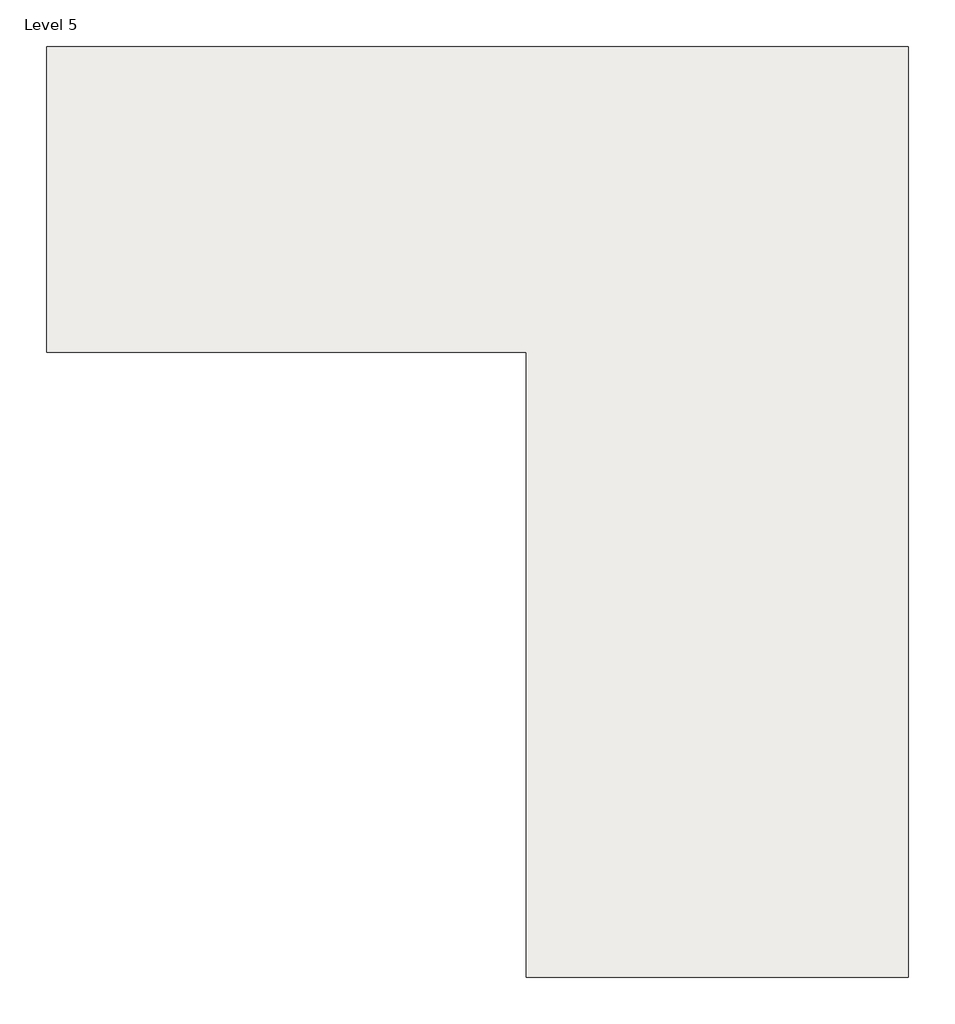
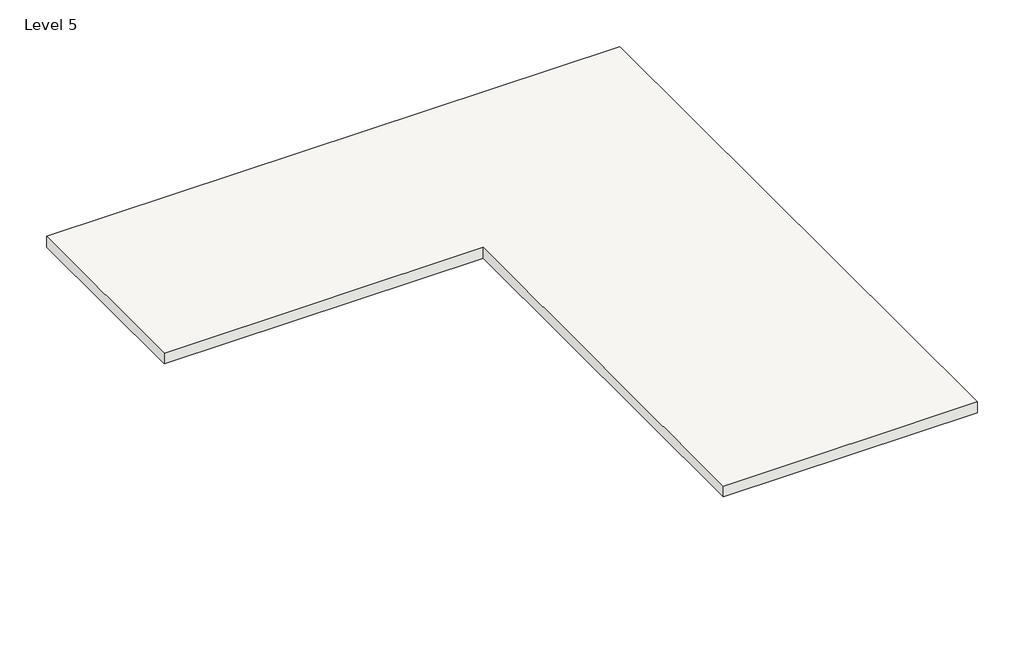
# One storey: 1 roof.
"""IFC4 building model written with IfcOpenShell, lengths in millimetres."""

from ifc_helpers import new_model, si_unit, frame, origin, place, context, project, spatial, polyline, outline, extrude, element, save

model = new_model("IFC4")

# Units and contexts
model_context = context("Model", 3, world=origin())
ifc_project = project(units=[si_unit("LENGTHUNIT", "METRE", prefix="MILLI")], contexts=[model_context])

# Site, building, storey
site = spatial("IfcSite", under=ifc_project)
building = spatial("IfcBuilding", under=site)
storey = spatial("IfcBuildingStorey", under=building, Name="Level 5", Elevation=14630.4)

# Roof
placement = place(None, origin())
element("IfcRoof", 1, ObjectType="Generic - 9\"", at=placement, inside=storey, context=model_context, shape_type="SweptSolid", body=[
    extrude(outline(polyline([(-16092.1624512, 7638.6627832), (-4573.2624512, 7638.6627832), (-4573.2624512, -4807.3372168), (-9680.4872956, -4807.3372168), (-9680.4872956, 3549.2627832), (-16092.1624512, 3549.2627832), (-16092.1624512, 7638.6627832)])), frame((0.0, 0.0, 14630.4), z_axis=(0.0, 0.0, 1.0), x_axis=(1.0, 0.0, 0.0)), (0.0, 0.0, 1.0), 228.6),
])

save(model, "model.ifc")

# Revit data of these elements
# Type "Generic - 9\""
#   Assembly Code = "B1020"
#   Layers, outside or top first: 0' - 9" no material (function 1)
# Element 1 (IfcRoof, "Generic - 9\"")
#   built-in parameter 1001705 = 48.75 (stored number, unit not read)
#   built-in parameter 1001710 = 33615
#   Phase Created = New Construction
#   Materials on its faces: "Default Roof", "Cherry"
# Materials
#   "Default Roof": colour RGB 88 101 114, transparency 0
#   "Cherry": class "Wood", colour RGB 226 177 128, transparency 0, Description = "Prunus Serotina", Cost = 0
